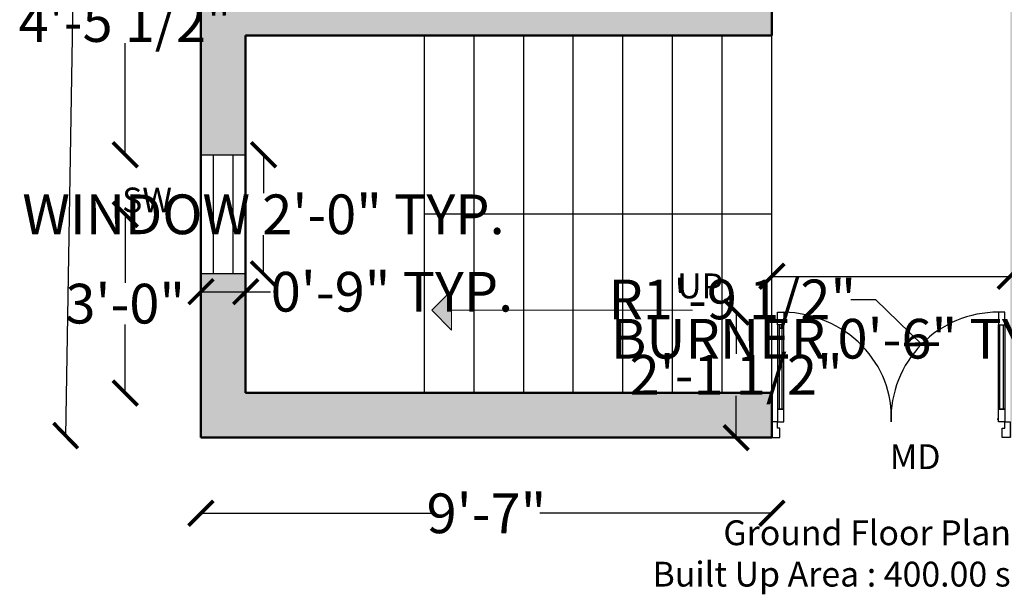
# Model space of a CAD drawing. Units: inches. Extents: x 2015 to 2400, y 1855 to 2156.
# Tile 1 of 3: x 2057 to 2255, y 1855 to 1971. Entities that reach past the tile are written whole.
import ezdxf

# ---------------------------------------------------------------- set-up
doc = ezdxf.new("R2010")
doc.units = ezdxf.units.IN
for name, color, linetype, lineweight in [('A-ANNO-DIMS', 2, 'Continuous', 18), ('A-ANNO-SYMB', 7, 'Continuous', 18), ('A-ANNO-TEXT', 7, 'Continuous', 25), ('A-WALL-PATT', 30, 'Continuous', 13), ('Door', 40, 'Continuous', 25), ('Steps', 50, 'Continuous', 25), ('Walls', 7, 'Continuous', 50), ('Windows', 150, 'Continuous', 25)]:
    doc.layers.add(name, color=color, linetype=linetype, lineweight=lineweight)
doc.layers.add('A-Glaz', color=92, linetype='Continuous')
doc.styles.get("Standard").update_dxf_attribs({"font": 'arial.ttf'})
doc.dimstyles.get("Standard").update_dxf_attribs({"dimtxt": 8, "dimasz": 5, "dimexe": 0.18, "dimexo": 0.0625, "dimgap": 0.09, "dimtad": 0, "dimtih": 1, "dimtoh": 1, "dimdec": 1, "dimzin": 0, "dimdsep": 46, "dimlunit": 4, "dimtxsty": 'Standard', "dimblk": 'ARCHTICK', "dimcen": 0.09, "dimse1": 1, "dimse2": 1, "dimadec": 0, "dimazin": 0, "dimtfac": 1, "dimtdec": 1, "dimtofl": 0, "dimtmove": 0, "dimatfit": 3, "dimfxl": 1, "dimtolj": 1, "dimtzin": 0, "dimarcsym": 0})

# ---------------------------------------------------------------- blocks, each defined once
blk = doc.blocks.new('A$C13CE0A17')
at = {"layer": 'A-Glaz'}
for p, q in [((0.01, 0.61), (0.01, 0.08)), ((0.03, 0.08), (0.03, 0.61))]:
    blk.add_line(p, q, dxfattribs=at)
blk.add_lwpolyline([(1.4, 0.08), (1.4, 0.61), (1.42, 0.61), (1.42, 0.08)], close=True, dxfattribs=at)
at = {"layer": 'Door'}
for p, q in [((0, 0.61), (0, 0.69)), ((0, 0.69), (0.04, 0.69)), ((0.04, 0.69), (0.04, 0.61)), ((0, 0.61), (0, 0.08)), ((0.04, 0.61), (0, 0.61)), ((0.04, 0.61), (0, 0.61)), ((0.03, 0.61), (0.01, 0.61)), ((0.04, 0.08), (0.04, 0.61)), ((0, 0.08), (0, 0)), ((0.04, 0.08), (0, 0.08)), ((0, 0.08), (0.04, 0.08)), ((0.01, 0.08), (0.03, 0.08)), ((0.04, 0), (0.04, 0.08)), ((-0.035, 0), (-0.035, -0.1)), ((0, 0), (-0.035, 0)), ((0, 0), (0.04, 0)), ((0, -0.04), (0, 0)), ((0.015, -0.04), (0, -0.04)), ((0.015, -0.05), (0.015, -0.04)), ((0.015, -0.1), (0.015, -0.05)), ((-0.035, -0.1), (0.015, -0.1))]:
    blk.add_line(p, q, dxfattribs=at)
for points in [[(1.39, 0.69), (1.39, 0.61), (1.43, 0.61), (1.43, 0.69)], [(1.39, 0.08), (1.39, 0.61), (1.43, 0.61), (1.43, 0.08)], [(1.39, 0), (1.39, 0.08), (1.43, 0.08), (1.43, 0)], [(1.43, 0), (1.465, 0), (1.465, -0.1), (1.415, -0.1), (1.415, -0.05), (1.415, -0.04), (1.43, -0.04)]]:
    blk.add_lwpolyline(points, close=True, dxfattribs=at)
blk.add_arc((1.3872, 0.017), 0.673, 89.76573, 181.44381, dxfattribs=at)
blk.add_ellipse((0.0389, 0.0511), major_axis=(0.6669, -0.1217), ratio=0.940794, start_param=0.11153, end_param=1.73917, dxfattribs=at)
blk = doc.blocks.new('_ArchTick')
at = {"color": 0, "linetype": 'ByBlock', "const_width": 0.15}
blk.add_lwpolyline([(-0.5, -0.5), (0.5, 0.5)], dxfattribs=at)
blk = doc.blocks.new('*D13')
at = {"layer": 'A-ANNO-DIMS', "color": 0, "lineweight": -2, "transparency": 16777216}
for p, q in [((2069.93, 2126.97), (2067.99, 2011.14)), ((2065.91, 1886.97), (2067.85, 2002.79))]:
    blk.add_line(p, q, dxfattribs=at)
at = {"layer": 'Defpoints', "color": 0, "transparency": 16777216}
for p in [(2093.14, 2126.58), (2065.91, 1886.97), (2089.12, 1886.58)]:
    blk.add_point(p, dxfattribs=at)
at = {"layer": 'A-ANNO-DIMS', "color": 0, "lineweight": -2, "transparency": 16777216, "xscale": 5, "yscale": 5, "zscale": 5}
for p, rotation in [((2069.93, 2126.97), 89.03988190259393), ((2065.91, 1886.97), 269.039881902594)]:
    blk.add_blockref('_ArchTick', p, dxfattribs=dict(at, rotation=rotation))
at = {"layer": 'A-ANNO-DIMS', "color": 0, "transparency": 16777216, "insert": (2067.92, 2006.97), "char_height": 8, "attachment_point": 5}
blk.add_mtext("\\A1;20'", dxfattribs=at)
blk = doc.blocks.new('WIN-24IN')
for p, q in [((2.5, 0), (2.5, 24)), ((6.5, 0), (6.5, 24))]:
    blk.add_line(p, q)
blk.add_lwpolyline([(0, 0), (0, 24), (9, 24), (9, 0)], close=True)
blk = doc.blocks.new('*D21')
at = {"layer": 'A-ANNO-DIMS', "color": 0, "lineweight": -2, "transparency": 16777216}
for p, q in [((2105.74, 1943.58), (2105.74, 1935.81)), ((2105.74, 1919.58), (2105.74, 1927.35))]:
    blk.add_line(p, q, dxfattribs=at)
at = {"layer": 'Defpoints', "color": 0, "transparency": 16777216}
for p in [(2102.14, 1943.58), (2105.74, 1943.58), (2102.14, 1919.58)]:
    blk.add_point(p, dxfattribs=at)
at = {"layer": 'A-ANNO-DIMS', "color": 0, "lineweight": -2, "transparency": 16777216, "xscale": 5, "yscale": 5, "zscale": 5}
for p, rotation in [((2105.74, 1943.58), 90), ((2105.74, 1919.58), 270)]:
    blk.add_blockref('_ArchTick', p, dxfattribs=dict(at, rotation=rotation))
at = {"layer": 'A-ANNO-DIMS', "color": 0, "transparency": 16777216, "insert": (2105.74, 1931.58), "char_height": 8, "attachment_point": 5}
blk.add_mtext('\\A1;WINDOW 2\'-0" TYP.', dxfattribs=at)
blk = doc.blocks.new('*D22')
at = {"layer": 'A-ANNO-DIMS', "color": 0, "lineweight": -2, "transparency": 16777216}
for p, q in [((2093.14, 1915.98), (2102.14, 1915.98)), ((2102.14, 1915.98), (2107.14, 1915.98))]:
    blk.add_line(p, q, dxfattribs=at)
at = {"layer": 'Defpoints', "color": 0, "transparency": 16777216}
for p in [(2093.14, 1919.58), (2102.14, 1919.58), (2102.14, 1915.98)]:
    blk.add_point(p, dxfattribs=at)
at = {"layer": 'A-ANNO-DIMS', "color": 0, "lineweight": -2, "transparency": 16777216, "xscale": 5, "yscale": 5, "zscale": 5, "rotation": 180}
blk.add_blockref('_ArchTick', (2093.14, 1915.98), dxfattribs=at)
at = {"layer": 'A-ANNO-DIMS', "color": 0, "lineweight": -2, "transparency": 16777216, "xscale": 5, "yscale": 5, "zscale": 5}
blk.add_blockref('_ArchTick', (2102.14, 1915.98), dxfattribs=at)
at = {"layer": 'A-ANNO-DIMS', "color": 0, "transparency": 16777216, "insert": (2131.61, 1915.98), "char_height": 8, "attachment_point": 5}
blk.add_mtext('\\A1;0\'-9" TYP.', dxfattribs=at)
blk = doc.blocks.new('*D23')
at = {"layer": 'A-ANNO-DIMS', "color": 0, "lineweight": -2, "transparency": 16777216}
for p, q in [((2277.38, 1906.51), (2272.38, 1906.51)), ((2283.36, 1906.51), (2277.38, 1906.51))]:
    blk.add_line(p, q, dxfattribs=at)
at = {"layer": 'Defpoints', "color": 0, "transparency": 16777216}
for p in [(2277.38, 1907.41), (2277.38, 1906.51), (2283.36, 1907.41)]:
    blk.add_point(p, dxfattribs=at)
at = {"layer": 'A-ANNO-DIMS', "color": 0, "lineweight": -2, "transparency": 16777216, "xscale": 5, "yscale": 5, "zscale": 5}
for p, rotation in [((2277.38, 1906.51), 179.9999999999891), ((2283.36, 1906.51), 359.9999999999891)]:
    blk.add_blockref('_ArchTick', p, dxfattribs=dict(at, rotation=rotation))
at = {"layer": 'A-ANNO-DIMS', "color": 0, "transparency": 16777216, "insert": (2222.93, 1906.51), "char_height": 8, "attachment_point": 5}
blk.add_mtext('\\A1;BURNER 0\'-6" TYP.', dxfattribs=at)
blk = doc.blocks.new('*D25')
at = {"layer": 'A-ANNO-DIMS', "color": 0, "lineweight": -2, "transparency": 16777216}
for p, q in [((2208.14, 1919.08), (2256.14, 1919.08)), ((2256.14, 1919.08), (2261.14, 1919.08))]:
    blk.add_line(p, q, dxfattribs=at)
at = {"layer": 'Defpoints', "color": 0, "transparency": 16777216}
for p in [(2256.14, 1919.08), (2208.14, 1911.88), (2256.14, 1911.88)]:
    blk.add_point(p, dxfattribs=at)
at = {"layer": 'A-ANNO-DIMS', "color": 0, "lineweight": -2, "transparency": 16777216, "xscale": 5, "yscale": 5, "zscale": 5, "rotation": 180}
blk.add_blockref('_ArchTick', (2208.14, 1919.08), dxfattribs=at)
at = {"layer": 'A-ANNO-DIMS', "color": 0, "lineweight": -2, "transparency": 16777216, "xscale": 5, "yscale": 5, "zscale": 5}
blk.add_blockref('_ArchTick', (2256.14, 1919.08), dxfattribs=at)
at = {"layer": 'A-ANNO-DIMS', "color": 0, "transparency": 16777216, "insert": (2292.14, 1919.08), "char_height": 8, "attachment_point": 5}
blk.add_mtext('\\A1;ENTRY 4\'-0"', dxfattribs=at)
blk = doc.blocks.new('*D26')
at = {"layer": 'A-ANNO-DIMS', "color": 0, "lineweight": -2, "transparency": 16777216}
for p, q in [((2200.94, 1911.88), (2200.94, 1903.46)), ((2200.94, 1886.58), (2200.94, 1895.01))]:
    blk.add_line(p, q, dxfattribs=at)
at = {"layer": 'Defpoints', "color": 0, "transparency": 16777216}
for p in [(2200.94, 1911.88), (2208.14, 1911.88), (2208.14, 1886.58)]:
    blk.add_point(p, dxfattribs=at)
at = {"layer": 'A-ANNO-DIMS', "color": 0, "lineweight": -2, "transparency": 16777216, "xscale": 5, "yscale": 5, "zscale": 5}
for p, rotation in [((2200.94, 1911.88), 90), ((2200.94, 1886.58), 270)]:
    blk.add_blockref('_ArchTick', p, dxfattribs=dict(at, rotation=rotation))
at = {"layer": 'A-ANNO-DIMS', "color": 0, "transparency": 16777216, "insert": (2200.94, 1899.23), "char_height": 8, "attachment_point": 5}
blk.add_mtext('\\A1;2\'-1 1/2"', dxfattribs=at)
blk = doc.blocks.new('*D37')
at = {"layer": 'A-ANNO-DIMS', "color": 0, "lineweight": -2, "transparency": 16777216}
for p, q in [((2093.14, 1871.33), (2139.92, 1871.33)), ((2208.14, 1871.33), (2161.36, 1871.33))]:
    blk.add_line(p, q, dxfattribs=at)
at = {"layer": 'Defpoints', "color": 0, "transparency": 16777216}
for p in [(2093.14, 1886.58), (2208.14, 1886.58), (2208.14, 1871.33)]:
    blk.add_point(p, dxfattribs=at)
at = {"layer": 'A-ANNO-DIMS', "color": 0, "lineweight": -2, "transparency": 16777216, "xscale": 5, "yscale": 5, "zscale": 5, "rotation": 180}
blk.add_blockref('_ArchTick', (2093.14, 1871.33), dxfattribs=at)
at = {"layer": 'A-ANNO-DIMS', "color": 0, "lineweight": -2, "transparency": 16777216, "xscale": 5, "yscale": 5, "zscale": 5}
blk.add_blockref('_ArchTick', (2208.14, 1871.33), dxfattribs=at)
at = {"layer": 'A-ANNO-DIMS', "color": 0, "transparency": 16777216, "insert": (2150.64, 1871.33), "char_height": 8, "attachment_point": 5}
blk.add_mtext('\\A1;9\'-7"', dxfattribs=at)
blk = doc.blocks.new('*D41')
at = {"layer": 'A-ANNO-DIMS', "color": 0, "lineweight": -2, "transparency": 16777216}
for p, q in [((2077.89, 1997.08), (2077.89, 1974.56)), ((2077.89, 1943.58), (2077.89, 1966.1))]:
    blk.add_line(p, q, dxfattribs=at)
at = {"layer": 'Defpoints', "color": 0, "transparency": 16777216}
for p in [(2077.89, 1997.08), (2093.14, 1997.08), (2093.14, 1943.58)]:
    blk.add_point(p, dxfattribs=at)
at = {"layer": 'A-ANNO-DIMS', "color": 0, "lineweight": -2, "transparency": 16777216, "xscale": 5, "yscale": 5, "zscale": 5}
for p, rotation in [((2077.89, 1997.08), 90), ((2077.89, 1943.58), 270)]:
    blk.add_blockref('_ArchTick', p, dxfattribs=dict(at, rotation=rotation))
at = {"layer": 'A-ANNO-DIMS', "color": 0, "transparency": 16777216, "insert": (2077.89, 1970.33), "char_height": 8, "attachment_point": 5}
blk.add_mtext('\\A1;4\'-5 1/2"', dxfattribs=at)
blk = doc.blocks.new('*D43')
at = {"layer": 'A-ANNO-DIMS', "color": 0, "lineweight": -2, "transparency": 16777216}
for p, q in [((2138.14, 2141.83), (2148.14, 2141.83)), ((2148.14, 2141.83), (2153.14, 2141.83))]:
    blk.add_line(p, q, dxfattribs=at)
at = {"layer": 'Defpoints', "color": 0, "transparency": 16777216}
for p in [(2148.14, 2141.83), (2138.14, 1895.58), (2148.14, 1895.58)]:
    blk.add_point(p, dxfattribs=at)
at = {"layer": 'A-ANNO-DIMS', "color": 0, "lineweight": -2, "transparency": 16777216, "xscale": 5, "yscale": 5, "zscale": 5, "rotation": 180}
blk.add_blockref('_ArchTick', (2138.14, 2141.83), dxfattribs=at)
at = {"layer": 'A-ANNO-DIMS', "color": 0, "lineweight": -2, "transparency": 16777216, "xscale": 5, "yscale": 5, "zscale": 5}
blk.add_blockref('_ArchTick', (2148.14, 2141.83), dxfattribs=at)
at = {"layer": 'A-ANNO-DIMS', "color": 0, "transparency": 16777216, "insert": (2166.97, 2141.83), "char_height": 8, "attachment_point": 5}
blk.add_mtext('\\A1;0\'-10"', dxfattribs=at)
blk = doc.blocks.new('*D44')
at = {"layer": 'A-ANNO-DIMS', "color": 0, "lineweight": -2, "transparency": 16777216}
for p, q in [((2077.89, 1931.58), (2077.89, 1917.76)), ((2077.89, 1895.58), (2077.89, 1909.4))]:
    blk.add_line(p, q, dxfattribs=at)
at = {"layer": 'Defpoints', "color": 0, "transparency": 16777216}
for p in [(2077.89, 1931.58), (2138.14, 1931.58), (2138.14, 1895.58)]:
    blk.add_point(p, dxfattribs=at)
at = {"layer": 'A-ANNO-DIMS', "color": 0, "lineweight": -2, "transparency": 16777216, "xscale": 5, "yscale": 5, "zscale": 5}
for p, rotation in [((2077.89, 1931.58), 90), ((2077.89, 1895.58), 270)]:
    blk.add_blockref('_ArchTick', p, dxfattribs=dict(at, rotation=rotation))
at = {"layer": 'A-ANNO-DIMS', "color": 0, "transparency": 16777216, "insert": (2077.89, 1913.58), "char_height": 8, "attachment_point": 5}
blk.add_mtext('\\A1;3\'-0"', dxfattribs=at)
blk = doc.blocks.new('*D55')
at = {"layer": 'A-ANNO-DIMS', "color": 0, "lineweight": -2, "transparency": 16777216}
for p, q in [((2224.03, 1914.43), (2229.03, 1914.43)), ((2229.03, 1914.43), (2238.26, 1905.39)), ((2253.56, 1890.32), (2253.74, 1890.32)), ((2253.65, 1890.23), (2253.65, 1890.41))]:
    blk.add_line(p, q, dxfattribs=at)
at = {"layer": 'Defpoints', "color": 0, "transparency": 16777216}
for p in [(2238.26, 1905.39), (2253.65, 1890.32)]:
    blk.add_point(p, dxfattribs=at)
at = {"layer": 'A-ANNO-DIMS', "color": 0, "lineweight": -2, "transparency": 16777216, "xscale": 5, "yscale": 5, "zscale": 5, "rotation": 315.6052518065289}
blk.add_blockref('_ArchTick', (2238.26, 1905.39), dxfattribs=at)
at = {"layer": 'A-ANNO-DIMS', "color": 0, "transparency": 16777216, "insert": (2200.16, 1914.43), "char_height": 8, "attachment_point": 5}
blk.add_mtext('\\A1;R1\'-9 1/2"', dxfattribs=at)

msp = doc.modelspace()

# ---------------------------------------------------------------- hatches: boundary and pattern name
at = {"layer": 'A-ANNO-SYMB'}
h = msp.add_hatch(color=256, dxfattribs=at)
h.dxf.hatch_style = 1
h.paths.add_polyline_path([(2143.63, 1916.25), (2139.63, 1912.25), (2143.63, 1908.25)])
at = {"layer": 'A-WALL-PATT'}
h = msp.add_hatch(color=256, dxfattribs=at)
h.dxf.hatch_style = 1
h.paths.add_polyline_path([(2236.14, 2126.58), (2093.14, 2126.58), (2093.14, 2111.58), (2102.14, 2111.58), (2102.14, 2111.85), (2102.14, 2117.58), (2204.14, 2117.58), (2204.14, 2005.56), (2208.14, 2005.56), (2208.14, 2117.58), (2236.14, 2117.58)])
h.paths.add_polyline_path([(2102.14, 2077.58), (2175.16, 2077.58), (2175.16, 2081.58), (2102.14, 2081.58), (2102.14, 2087.58), (2093.14, 2087.58), (2093.14, 2057.08), (2102.14, 2057.08), (2102.14, 2057.96)], flags=17)
h.paths.add_polyline_path([(2208.14, 1976.58), (2203.68, 1976.58), (2174.71, 1976.58), (2102.14, 1976.58), (2102.14, 1997.08), (2093.14, 1997.08), (2093.14, 1943.58), (2102.14, 1943.58), (2102.14, 1967.58), (2208.14, 1967.58)])
h.paths.add_polyline_path([(2260.14, 1976.58), (2256.14, 1976.58), (2256.14, 1886.58), (2262.02, 1886.58), (2262.02, 1895.58), (2260.14, 1895.58)])
h.paths.add_polyline_path([(2208.14, 1895.58), (2102.14, 1895.58), (2102.14, 1919.58), (2093.14, 1919.58), (2093.14, 1886.58), (2208.14, 1886.58)])

# ---------------------------------------------------------------- linework, layer by layer
at = {"layer": 'A-ANNO-SYMB'}
for p, q in [((2139.63, 1912.25), (2143.63, 1916.25)), ((2143.63, 1908.25), (2143.63, 1916.25)), ((2139.63, 1912.25), (2143.63, 1908.25)), ((2192.13, 1912.25), (2143.63, 1912.25))]:
    msp.add_line(p, q, dxfattribs=at)
at = {"layer": 'Steps'}
for p, q in [((2138.14, 1895.58), (2138.14, 1967.58)), ((2148.14, 1895.58), (2148.14, 1967.58)), ((2158.14, 1895.58), (2158.14, 1967.58)), ((2168.14, 1895.58), (2168.14, 1967.58)), ((2178.14, 1895.58), (2178.14, 1967.58)), ((2188.14, 1895.58), (2188.14, 1967.58)), ((2198.14, 1895.58), (2198.14, 1967.58)), ((2208.14, 1895.58), (2208.14, 1967.58)), ((2208.14, 1931.58), (2138.14, 1931.58))]:
    msp.add_line(p, q, dxfattribs=at)
at = {"layer": 'Walls'}
for p, q in [((2093.14, 2126.58), (2093.14, 1886.58)), ((2208.14, 1976.58), (2208.14, 1967.58)), ((2102.14, 1967.58), (2208.14, 1967.58)), ((2102.14, 1967.58), (2102.14, 1895.58)), ((2102.14, 1895.58), (2208.14, 1895.58)), ((2208.14, 1895.58), (2208.14, 1886.58)), ((2093.14, 1886.58), (2208.14, 1886.58))]:
    msp.add_line(p, q, dxfattribs=at)

# ---------------------------------------------------------------- block references
at = {"layer": 'Door', "xscale": 31.99999999999989, "yscale": 31.99999999999989, "zscale": 31.99999999999989}
msp.add_blockref('A$C13CE0A17', (2209.26, 1889.78), dxfattribs=at)
at = {"layer": 'Windows'}
msp.add_blockref('WIN-24IN', (2093.14, 1919.58), dxfattribs=at)

# ---------------------------------------------------------------- texts
at = {"layer": 'A-ANNO-TEXT', "char_height": 5, "attachment_point": 1}
for s, width, heights, insert in [('\\pxqc;SW', 31.0576, [0], (2066.75, 1936.97)), ('\\pxqc;UP', 31.0576, [0], (2178.14, 1919.66)), ('\\pxqc;MD', 31.0576, [0], (2221.46, 1885.24)), ('\\pxqc;Ground Floor Plan\\PBuilt Up Area : 400.00 sq. ft.', 115.2426, [17.51], (2169.7, 1869.91))]:
    msp.add_mtext_dynamic_manual_height_columns(s, width=width, gutter_width=12.5, heights=heights, dxfattribs=dict(at, insert=insert))

# ---------------------------------------------------------------- dimensions: what is measured, and where the dimension line sits
at = {"layer": 'A-ANNO-DIMS'}
for base, p1, p2, picture, middle in [((2148.14, 2141.83), (2138.14, 1895.58), (2148.14, 1895.58), '*D43', (2166.97, 2141.83)), ((2208.14, 1871.33), (2093.14, 1886.58), (2208.14, 1886.58), '*D37', (2150.64, 1871.33))]:
    dim = msp.add_linear_dim(base=base, p1=p1, p2=p2, dimstyle='Standard', override={"dimdec": 1, "dimlfac": 1, "dimrnd": 0, "dimzin": 1, "dimdsep": 46, "dimlunit": 4, "dimfrac": 2}, dxfattribs=at)
    dim.commit()
    dim.dimension.update_dxf_attribs({"geometry": picture, "text_midpoint": middle})
dim = msp.add_aligned_dim(p1=(2093.14, 2126.58), p2=(2089.12, 1886.58), distance=-23.21, dimstyle='Standard', override={"dimclrd": 0, "dimclre": 0, "dimclrt": 0}, dxfattribs=at)
dim.commit()
dim.dimension.update_dxf_attribs({"geometry": '*D13', "text_midpoint": (2067.92, 2006.97)})
for base, p1, p2, picture, middle in [((2077.89, 1997.08), (2093.14, 1943.58), (2093.14, 1997.08), '*D41', (2077.89, 1970.33)), ((2077.89, 1931.58), (2138.14, 1895.58), (2138.14, 1931.58), '*D44', (2077.89, 1913.58)), ((2200.94, 1911.88), (2208.14, 1886.58), (2208.14, 1911.88), '*D26', (2200.94, 1899.23))]:
    dim = msp.add_linear_dim(base=base, p1=p1, p2=p2, angle=90, dimstyle='Standard', override={"dimdec": 1, "dimlfac": 1, "dimrnd": 0, "dimzin": 1, "dimdsep": 46, "dimlunit": 4, "dimfrac": 2}, dxfattribs=at)
    dim.commit()
    dim.dimension.update_dxf_attribs({"geometry": picture, "text_midpoint": middle})
for base, p1, p2, angle, text, picture, middle in [((2105.74, 1943.58), (2102.14, 1919.58), (2102.14, 1943.58), 90, 'WINDOW <> TYP.', '*D21', (2105.74, 1931.58)), ((2277.38, 1906.51), (2283.36, 1907.41), (2277.38, 1907.41), 180, 'BURNER <> TYP.', '*D23', (2222.93, 1906.51))]:
    dim = msp.add_linear_dim(base=base, p1=p1, p2=p2, angle=angle, text=text, dimstyle='Standard', override={"dimdec": 1, "dimlfac": 1, "dimrnd": 0, "dimzin": 1, "dimdsep": 46, "dimlunit": 4, "dimfrac": 2}, dxfattribs=at)
    dim.commit()
    dim.dimension.update_dxf_attribs({"geometry": picture, "text_midpoint": middle})
for base, p1, p2, text, picture, middle in [((2256.14, 1919.08), (2208.14, 1911.88), (2256.14, 1911.88), 'ENTRY <>', '*D25', (2292.14, 1919.08)), ((2102.14, 1915.98), (2093.14, 1919.58), (2102.14, 1919.58), '<> TYP.', '*D22', (2131.61, 1915.98))]:
    dim = msp.add_linear_dim(base=base, p1=p1, p2=p2, text=text, dimstyle='Standard', override={"dimdec": 1, "dimlfac": 1, "dimrnd": 0, "dimzin": 1, "dimdsep": 46, "dimlunit": 4, "dimfrac": 2}, dxfattribs=at)
    dim.commit()
    dim.dimension.update_dxf_attribs({"geometry": picture, "text_midpoint": middle})
dim = msp.add_radius_dim(center=(2253.65, 1890.32), mpoint=(2238.26, 1905.39), dimstyle='Standard', override={"dimdec": 1, "dimlfac": 1, "dimrnd": 0, "dimzin": 1, "dimdsep": 46, "dimlunit": 4, "dimfrac": 2}, dxfattribs=at)
dim.commit()
dim.dimension.update_dxf_attribs({"geometry": '*D55', "text_midpoint": (2200.16, 1914.43), "dimtype": 164})

doc.saveas('drawing.dxf')
